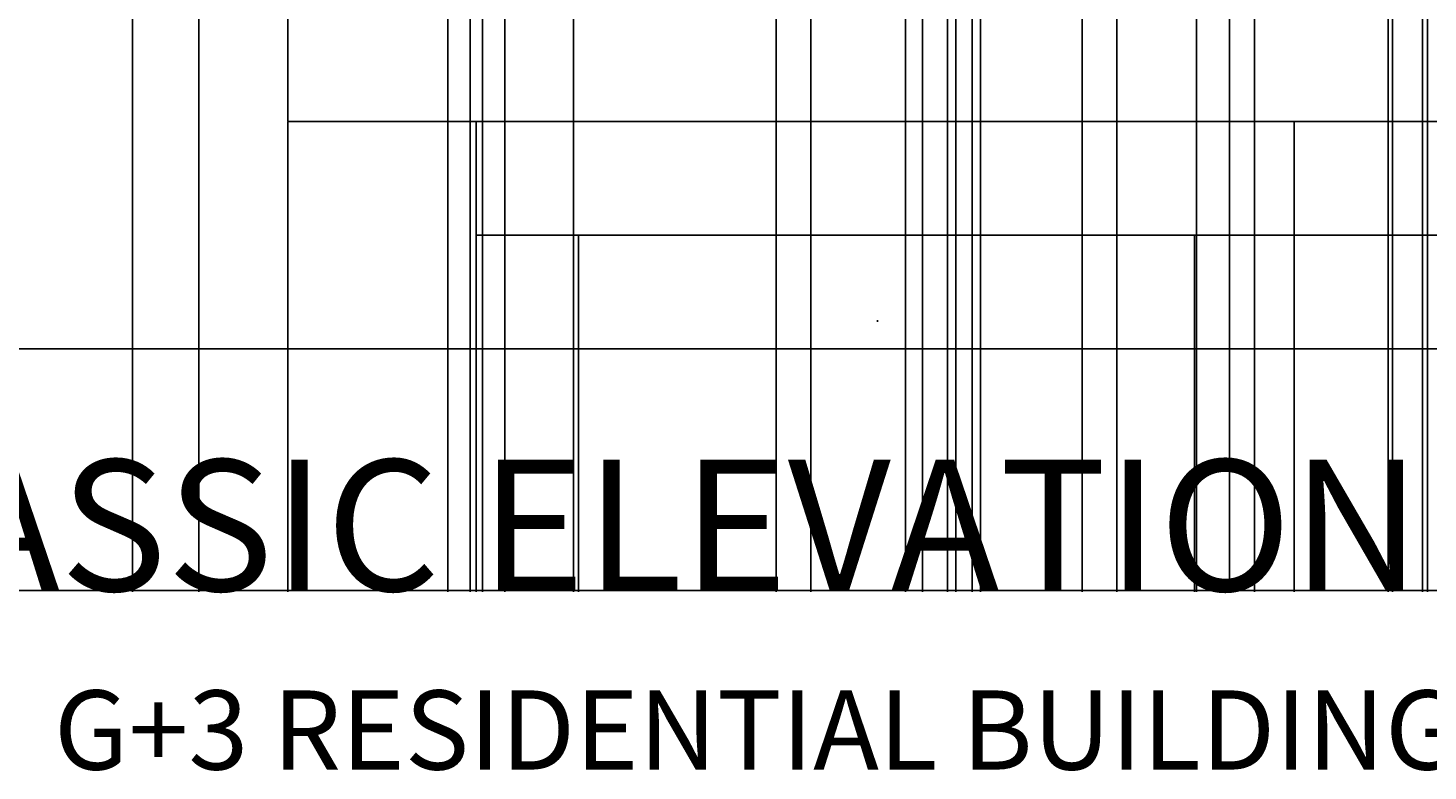
# Model space of a CAD drawing. Units: inches. Extents: x -14 to 375, y -86 to 549.
# Tile 2 of 12: x 122 to 290, y -86 to 4. Entities that reach past the tile are written whole.
import ezdxf

# ---------------------------------------------------------------- set-up
doc = ezdxf.new("R2010")
doc.units = ezdxf.units.IN
doc.header["$MEASUREMENT"] = 0
for name, color, linetype, lineweight in [('A-ANNO-DIMS', 2, 'Continuous', 18), ('A-ANNO-TEXT', 7, 'Continuous', 25), ('A-ELEV', 7, 'Continuous', 25)]:
    doc.layers.add(name, color=color, linetype=linetype, lineweight=lineweight)
doc.styles.get("Standard").update_dxf_attribs({"font": 'arial.ttf'})
doc.dimstyles.get("Standard").update_dxf_attribs({"dimtxt": 0.18, "dimasz": 0.18, "dimexe": 0.18, "dimexo": 0.0625, "dimgap": 0.09, "dimtad": 0, "dimtih": 1, "dimtoh": 1, "dimdec": 4, "dimzin": 0, "dimdsep": 46, "dimtxsty": 'Standard', "dimcen": 0.09, "dimadec": 0, "dimazin": 0, "dimtfac": 1, "dimtdec": 4, "dimtofl": 0, "dimtmove": 0, "dimatfit": 3, "dimfxl": 1, "dimtolj": 1, "dimtzin": 0, "dimarcsym": 0})

# ---------------------------------------------------------------- blocks, each defined once
blk = doc.blocks.new('*D4')
at = {"layer": 'A-ANNO-DIMS', "color": 0, "lineweight": -2, "transparency": 16777216}
for p, q in [((15.4, -35.17), (15.4, -64.39)), ((345.26, -35.17), (345.26, -64.39)), ((15.58, -64.21), (179.87, -64.21)), ((345.08, -64.21), (180.8, -64.21))]:
    blk.add_line(p, q, dxfattribs=at)
at = {"layer": 'A-ANNO-DIMS', "color": 0, "transparency": 16777216}
for points in [[(15.58, -64.18), (15.58, -64.24), (15.4, -64.21)], [(345.08, -64.18), (345.08, -64.24), (345.26, -64.21)]]:
    blk.add_solid(points, dxfattribs=at)
at = {"layer": 'Defpoints', "color": 0, "transparency": 16777216}
for p in [(15.4, -35.11), (345.26, -35.11), (345.26, -64.21)]:
    blk.add_point(p, dxfattribs=at)
at = {"layer": 'A-ANNO-DIMS', "color": 0, "transparency": 16777216, "insert": (180.33, -64.21), "char_height": 0.18, "attachment_point": 5}
blk.add_mtext('\\A1;329.86', dxfattribs=at)
blk = doc.blocks.new('*D42')
at = {"layer": 'A-ANNO-DIMS', "color": 0, "lineweight": -2, "transparency": 16777216}
for p, q in [((142.23, 270.64), (142.23, -64.39)), ((134.23, 262.64), (134.23, -64.39)), ((134.41, -64.21), (138.08, -64.21)), ((142.05, -64.21), (138.38, -64.21))]:
    blk.add_line(p, q, dxfattribs=at)
at = {"layer": 'A-ANNO-DIMS', "color": 0, "transparency": 16777216}
for points in [[(134.41, -64.18), (134.41, -64.24), (134.23, -64.21)], [(142.05, -64.18), (142.05, -64.24), (142.23, -64.21)]]:
    blk.add_solid(points, dxfattribs=at)
at = {"layer": 'Defpoints', "color": 0, "transparency": 16777216}
for p in [(142.23, 270.71), (134.23, 262.71), (142.23, -64.21)]:
    blk.add_point(p, dxfattribs=at)
at = {"layer": 'A-ANNO-DIMS', "color": 0, "transparency": 16777216, "insert": (138.23, -64.21), "char_height": 0.18, "attachment_point": 5}
blk.add_mtext('\\A1;8', dxfattribs=at)
blk = doc.blocks.new('*D43')
at = {"layer": 'A-ANNO-DIMS', "color": 0, "lineweight": -2, "transparency": 16777216}
for p, q in [((142.23, 270.64), (142.23, -64.39)), ((305.63, 270.64), (305.63, -64.39)), ((142.41, -64.21), (223.55, -64.21)), ((305.45, -64.21), (224.32, -64.21))]:
    blk.add_line(p, q, dxfattribs=at)
at = {"layer": 'A-ANNO-DIMS', "color": 0, "transparency": 16777216}
for points in [[(142.41, -64.18), (142.41, -64.24), (142.23, -64.21)], [(305.45, -64.18), (305.45, -64.24), (305.63, -64.21)]]:
    blk.add_solid(points, dxfattribs=at)
at = {"layer": 'Defpoints', "color": 0, "transparency": 16777216}
for p in [(142.23, 270.71), (305.63, 270.71), (305.63, -64.21)]:
    blk.add_point(p, dxfattribs=at)
at = {"layer": 'A-ANNO-DIMS', "color": 0, "transparency": 16777216, "insert": (223.93, -64.21), "char_height": 0.18, "attachment_point": 5}
blk.add_mtext('\\A1;163.4', dxfattribs=at)
blk = doc.blocks.new('*D45')
at = {"layer": 'A-ANNO-DIMS', "color": 0, "lineweight": -2, "transparency": 16777216}
for p, q in [((142.23, 306.64), (142.23, -64.39)), ((174.92, 306.64), (174.92, -64.39)), ((142.41, -64.21), (158.19, -64.21)), ((174.74, -64.21), (158.97, -64.21))]:
    blk.add_line(p, q, dxfattribs=at)
at = {"layer": 'A-ANNO-DIMS', "color": 0, "transparency": 16777216}
for points in [[(142.41, -64.18), (142.41, -64.24), (142.23, -64.21)], [(174.74, -64.18), (174.74, -64.24), (174.92, -64.21)]]:
    blk.add_solid(points, dxfattribs=at)
at = {"layer": 'Defpoints', "color": 0, "transparency": 16777216}
for p in [(142.23, 306.71), (174.92, 306.71), (174.92, -64.21)]:
    blk.add_point(p, dxfattribs=at)
at = {"layer": 'A-ANNO-DIMS', "color": 0, "transparency": 16777216, "insert": (158.58, -64.21), "char_height": 0.18, "attachment_point": 5}
blk.add_mtext('\\A1;32.69', dxfattribs=at)
blk = doc.blocks.new('*D46')
at = {"layer": 'A-ANNO-DIMS', "color": 0, "lineweight": -2, "transparency": 16777216}
for p, q in [((174.92, 306.64), (174.92, -64.39)), ((179.09, 306.64), (179.09, -64.39)), ((175.1, -64.21), (176.68, -64.21)), ((178.91, -64.21), (177.33, -64.21))]:
    blk.add_line(p, q, dxfattribs=at)
at = {"layer": 'A-ANNO-DIMS', "color": 0, "transparency": 16777216}
for points in [[(175.1, -64.18), (175.1, -64.24), (174.92, -64.21)], [(178.91, -64.18), (178.91, -64.24), (179.09, -64.21)]]:
    blk.add_solid(points, dxfattribs=at)
at = {"layer": 'Defpoints', "color": 0, "transparency": 16777216}
for p in [(174.92, 306.71), (179.09, 306.71), (179.09, -64.21)]:
    blk.add_point(p, dxfattribs=at)
at = {"layer": 'A-ANNO-DIMS', "color": 0, "transparency": 16777216, "insert": (177.01, -64.21), "char_height": 0.18, "attachment_point": 5}
blk.add_mtext('\\A1;4.17', dxfattribs=at)
blk = doc.blocks.new('*D47')
at = {"layer": 'A-ANNO-DIMS', "color": 0, "lineweight": -2, "transparency": 16777216}
for p, q in [((179.09, 306.64), (179.09, -64.39)), ((211.78, 306.64), (211.78, -64.39)), ((179.27, -64.21), (195.04, -64.21)), ((211.6, -64.21), (195.83, -64.21))]:
    blk.add_line(p, q, dxfattribs=at)
at = {"layer": 'A-ANNO-DIMS', "color": 0, "transparency": 16777216}
for points in [[(179.27, -64.18), (179.27, -64.24), (179.09, -64.21)], [(211.6, -64.18), (211.6, -64.24), (211.78, -64.21)]]:
    blk.add_solid(points, dxfattribs=at)
at = {"layer": 'Defpoints', "color": 0, "transparency": 16777216}
for p in [(179.09, 306.71), (211.78, 306.71), (211.78, -64.21)]:
    blk.add_point(p, dxfattribs=at)
at = {"layer": 'A-ANNO-DIMS', "color": 0, "transparency": 16777216, "insert": (195.44, -64.21), "char_height": 0.18, "attachment_point": 5}
blk.add_mtext('\\A1;32.69', dxfattribs=at)
blk = doc.blocks.new('*D48')
at = {"layer": 'A-ANNO-DIMS', "color": 0, "lineweight": -2, "transparency": 16777216}
for p, q in [((211.78, 306.64), (211.78, -64.39)), ((215.95, 306.64), (215.95, -64.39)), ((211.96, -64.21), (213.54, -64.21)), ((215.77, -64.21), (214.19, -64.21))]:
    blk.add_line(p, q, dxfattribs=at)
at = {"layer": 'A-ANNO-DIMS', "color": 0, "transparency": 16777216}
for points in [[(211.96, -64.18), (211.96, -64.24), (211.78, -64.21)], [(215.77, -64.18), (215.77, -64.24), (215.95, -64.21)]]:
    blk.add_solid(points, dxfattribs=at)
at = {"layer": 'Defpoints', "color": 0, "transparency": 16777216}
for p in [(211.78, 306.71), (215.95, 306.71), (215.95, -64.21)]:
    blk.add_point(p, dxfattribs=at)
at = {"layer": 'A-ANNO-DIMS', "color": 0, "transparency": 16777216, "insert": (213.86, -64.21), "char_height": 0.18, "attachment_point": 5}
blk.add_mtext('\\A1;4.17', dxfattribs=at)
blk = doc.blocks.new('*D49')
at = {"layer": 'A-ANNO-DIMS', "color": 0, "lineweight": -2, "transparency": 16777216}
for p, q in [((215.95, 306.64), (215.95, -64.39)), ((248.64, 306.64), (248.64, -64.39)), ((216.13, -64.21), (231.9, -64.21)), ((248.46, -64.21), (232.69, -64.21))]:
    blk.add_line(p, q, dxfattribs=at)
at = {"layer": 'A-ANNO-DIMS', "color": 0, "transparency": 16777216}
for points in [[(216.13, -64.18), (216.13, -64.24), (215.95, -64.21)], [(248.46, -64.18), (248.46, -64.24), (248.64, -64.21)]]:
    blk.add_solid(points, dxfattribs=at)
at = {"layer": 'Defpoints', "color": 0, "transparency": 16777216}
for p in [(215.95, 306.71), (248.64, 306.71), (248.64, -64.21)]:
    blk.add_point(p, dxfattribs=at)
at = {"layer": 'A-ANNO-DIMS', "color": 0, "transparency": 16777216, "insert": (232.29, -64.21), "char_height": 0.18, "attachment_point": 5}
blk.add_mtext('\\A1;32.69', dxfattribs=at)
blk = doc.blocks.new('*D50')
at = {"layer": 'A-ANNO-DIMS', "color": 0, "lineweight": -2, "transparency": 16777216}
for p, q in [((248.64, 306.64), (248.64, -64.39)), ((252.81, 306.64), (252.81, -64.39)), ((248.82, -64.21), (250.39, -64.21)), ((252.63, -64.21), (251.05, -64.21))]:
    blk.add_line(p, q, dxfattribs=at)
at = {"layer": 'A-ANNO-DIMS', "color": 0, "transparency": 16777216}
for points in [[(248.82, -64.18), (248.82, -64.24), (248.64, -64.21)], [(252.63, -64.18), (252.63, -64.24), (252.81, -64.21)]]:
    blk.add_solid(points, dxfattribs=at)
at = {"layer": 'Defpoints', "color": 0, "transparency": 16777216}
for p in [(248.64, 306.71), (252.81, 306.71), (252.81, -64.21)]:
    blk.add_point(p, dxfattribs=at)
at = {"layer": 'A-ANNO-DIMS', "color": 0, "transparency": 16777216, "insert": (250.72, -64.21), "char_height": 0.18, "attachment_point": 5}
blk.add_mtext('\\A1;4.17', dxfattribs=at)
blk = doc.blocks.new('*D51')
at = {"layer": 'A-ANNO-DIMS', "color": 0, "lineweight": -2, "transparency": 16777216}
for p, q in [((252.81, 306.64), (252.81, -64.39)), ((285.5, 306.64), (285.5, -64.39)), ((252.99, -64.21), (268.76, -64.21)), ((285.32, -64.21), (269.54, -64.21))]:
    blk.add_line(p, q, dxfattribs=at)
at = {"layer": 'A-ANNO-DIMS', "color": 0, "transparency": 16777216}
for points in [[(252.99, -64.18), (252.99, -64.24), (252.81, -64.21)], [(285.32, -64.18), (285.32, -64.24), (285.5, -64.21)]]:
    blk.add_solid(points, dxfattribs=at)
at = {"layer": 'Defpoints', "color": 0, "transparency": 16777216}
for p in [(252.81, 306.71), (285.5, 306.71), (285.5, -64.21)]:
    blk.add_point(p, dxfattribs=at)
at = {"layer": 'A-ANNO-DIMS', "color": 0, "transparency": 16777216, "insert": (269.15, -64.21), "char_height": 0.18, "attachment_point": 5}
blk.add_mtext('\\A1;32.69', dxfattribs=at)
blk = doc.blocks.new('*D52')
at = {"layer": 'A-ANNO-DIMS', "color": 0, "lineweight": -2, "transparency": 16777216}
for p, q in [((285.5, 306.64), (285.5, -64.39)), ((289.66, 306.64), (289.66, -64.39)), ((285.68, -64.21), (287.25, -64.21)), ((289.48, -64.21), (287.91, -64.21))]:
    blk.add_line(p, q, dxfattribs=at)
at = {"layer": 'A-ANNO-DIMS', "color": 0, "transparency": 16777216}
for points in [[(285.68, -64.18), (285.68, -64.24), (285.5, -64.21)], [(289.48, -64.18), (289.48, -64.24), (289.66, -64.21)]]:
    blk.add_solid(points, dxfattribs=at)
at = {"layer": 'Defpoints', "color": 0, "transparency": 16777216}
for p in [(285.5, 306.71), (289.66, 306.71), (289.66, -64.21)]:
    blk.add_point(p, dxfattribs=at)
at = {"layer": 'A-ANNO-DIMS', "color": 0, "transparency": 16777216, "insert": (287.58, -64.21), "char_height": 0.18, "attachment_point": 5}
blk.add_mtext('\\A1;4.17', dxfattribs=at)
blk = doc.blocks.new('*D57')
at = {"layer": 'A-ANNO-DIMS', "color": 0, "lineweight": -2, "transparency": 16777216}
for p, q in [((229.41, 340.38), (229.41, -64.39)), ((232.41, 340.38), (232.41, -64.39)), ((229.59, -64.21), (230.76, -64.21)), ((232.23, -64.21), (231.06, -64.21))]:
    blk.add_line(p, q, dxfattribs=at)
at = {"layer": 'A-ANNO-DIMS', "color": 0, "transparency": 16777216}
for points in [[(229.59, -64.18), (229.59, -64.24), (229.41, -64.21)], [(232.23, -64.18), (232.23, -64.24), (232.41, -64.21)]]:
    blk.add_solid(points, dxfattribs=at)
at = {"layer": 'Defpoints', "color": 0, "transparency": 16777216}
for p in [(229.41, 340.44), (232.41, 340.44), (232.41, -64.21)]:
    blk.add_point(p, dxfattribs=at)
at = {"layer": 'A-ANNO-DIMS', "color": 0, "transparency": 16777216, "insert": (230.91, -64.21), "char_height": 0.18, "attachment_point": 5}
blk.add_mtext('\\A1;3', dxfattribs=at)
blk = doc.blocks.new('*D58')
at = {"layer": 'A-ANNO-DIMS', "color": 0, "lineweight": -2, "transparency": 16777216}
for p, q in [((232.41, 340.38), (232.41, -64.39)), ((236.41, 340.38), (236.41, -64.39)), ((232.59, -64.21), (234.26, -64.21)), ((236.23, -64.21), (234.56, -64.21))]:
    blk.add_line(p, q, dxfattribs=at)
at = {"layer": 'A-ANNO-DIMS', "color": 0, "transparency": 16777216}
for points in [[(232.59, -64.18), (232.59, -64.24), (232.41, -64.21)], [(236.23, -64.18), (236.23, -64.24), (236.41, -64.21)]]:
    blk.add_solid(points, dxfattribs=at)
at = {"layer": 'Defpoints', "color": 0, "transparency": 16777216}
for p in [(232.41, 340.44), (236.41, 340.44), (236.41, -64.21)]:
    blk.add_point(p, dxfattribs=at)
at = {"layer": 'A-ANNO-DIMS', "color": 0, "transparency": 16777216, "insert": (234.41, -64.21), "char_height": 0.18, "attachment_point": 5}
blk.add_mtext('\\A1;4', dxfattribs=at)
blk = doc.blocks.new('*D59')
at = {"layer": 'A-ANNO-DIMS', "color": 0, "lineweight": -2, "transparency": 16777216}
for p, q in [((236.41, 340.38), (236.41, -64.39)), ((262.41, 340.38), (262.41, -64.39)), ((236.59, -64.21), (249.19, -64.21)), ((262.23, -64.21), (249.63, -64.21))]:
    blk.add_line(p, q, dxfattribs=at)
at = {"layer": 'A-ANNO-DIMS', "color": 0, "transparency": 16777216}
for points in [[(236.59, -64.18), (236.59, -64.24), (236.41, -64.21)], [(262.23, -64.18), (262.23, -64.24), (262.41, -64.21)]]:
    blk.add_solid(points, dxfattribs=at)
at = {"layer": 'Defpoints', "color": 0, "transparency": 16777216}
for p in [(236.41, 340.44), (262.41, 340.44), (262.41, -64.21)]:
    blk.add_point(p, dxfattribs=at)
at = {"layer": 'A-ANNO-DIMS', "color": 0, "transparency": 16777216, "insert": (249.41, -64.21), "char_height": 0.18, "attachment_point": 5}
blk.add_mtext('\\A1;26', dxfattribs=at)
blk = doc.blocks.new('*D60')
at = {"layer": 'A-ANNO-DIMS', "color": 0, "lineweight": -2, "transparency": 16777216}
for p, q in [((262.41, 340.38), (262.41, -64.39)), ((266.41, 340.38), (266.41, -64.39)), ((262.59, -64.21), (264.26, -64.21)), ((266.23, -64.21), (264.56, -64.21))]:
    blk.add_line(p, q, dxfattribs=at)
at = {"layer": 'A-ANNO-DIMS', "color": 0, "transparency": 16777216}
for points in [[(262.59, -64.18), (262.59, -64.24), (262.41, -64.21)], [(266.23, -64.18), (266.23, -64.24), (266.41, -64.21)]]:
    blk.add_solid(points, dxfattribs=at)
at = {"layer": 'Defpoints', "color": 0, "transparency": 16777216}
for p in [(262.41, 340.44), (266.41, 340.44), (266.41, -64.21)]:
    blk.add_point(p, dxfattribs=at)
at = {"layer": 'A-ANNO-DIMS', "color": 0, "transparency": 16777216, "insert": (264.41, -64.21), "char_height": 0.18, "attachment_point": 5}
blk.add_mtext('\\A1;4', dxfattribs=at)
blk = doc.blocks.new('*D61')
at = {"layer": 'A-ANNO-DIMS', "color": 0, "lineweight": -2, "transparency": 16777216}
for p, q in [((266.41, 340.38), (266.41, -64.39)), ((269.41, 340.38), (269.41, -64.39)), ((266.59, -64.21), (267.76, -64.21)), ((269.23, -64.21), (268.06, -64.21))]:
    blk.add_line(p, q, dxfattribs=at)
at = {"layer": 'A-ANNO-DIMS', "color": 0, "transparency": 16777216}
for points in [[(266.59, -64.18), (266.59, -64.24), (266.41, -64.21)], [(269.23, -64.18), (269.23, -64.24), (269.41, -64.21)]]:
    blk.add_solid(points, dxfattribs=at)
at = {"layer": 'Defpoints', "color": 0, "transparency": 16777216}
for p in [(266.41, 340.44), (269.41, 340.44), (269.41, -64.21)]:
    blk.add_point(p, dxfattribs=at)
at = {"layer": 'A-ANNO-DIMS', "color": 0, "transparency": 16777216, "insert": (267.91, -64.21), "char_height": 0.18, "attachment_point": 5}
blk.add_mtext('\\A1;3', dxfattribs=at)
blk = doc.blocks.new('*D71')
at = {"layer": 'A-ANNO-DIMS', "color": 0, "lineweight": -2, "transparency": 16777216}
for p, q in [((233.41, 167.91), (233.41, -64.39)), ((235.41, 167.91), (235.41, -64.39)), ((233.59, -64.21), (234.26, -64.21)), ((235.23, -64.21), (234.56, -64.21))]:
    blk.add_line(p, q, dxfattribs=at)
at = {"layer": 'A-ANNO-DIMS', "color": 0, "transparency": 16777216}
for points in [[(233.59, -64.18), (233.59, -64.24), (233.41, -64.21)], [(235.23, -64.18), (235.23, -64.24), (235.41, -64.21)]]:
    blk.add_solid(points, dxfattribs=at)
at = {"layer": 'Defpoints', "color": 0, "transparency": 16777216}
for p in [(233.41, 167.97), (235.41, 167.97), (235.41, -64.21)]:
    blk.add_point(p, dxfattribs=at)
at = {"layer": 'A-ANNO-DIMS', "color": 0, "transparency": 16777216, "insert": (234.41, -64.21), "char_height": 0.18, "attachment_point": 5}
blk.add_mtext('\\A1;2', dxfattribs=at)
blk = doc.blocks.new('*D74')
at = {"layer": 'A-ANNO-DIMS', "color": 0, "lineweight": -2, "transparency": 16777216}
for p, q in [((142.23, 125.9), (142.23, -64.39)), ((134.23, 117.9), (134.23, -64.39)), ((134.41, -64.21), (138.08, -64.21)), ((142.05, -64.21), (138.38, -64.21))]:
    blk.add_line(p, q, dxfattribs=at)
at = {"layer": 'A-ANNO-DIMS', "color": 0, "transparency": 16777216}
for points in [[(134.41, -64.18), (134.41, -64.24), (134.23, -64.21)], [(142.05, -64.18), (142.05, -64.24), (142.23, -64.21)]]:
    blk.add_solid(points, dxfattribs=at)
at = {"layer": 'Defpoints', "color": 0, "transparency": 16777216}
for p in [(142.23, 125.96), (134.23, 117.96), (142.23, -64.21)]:
    blk.add_point(p, dxfattribs=at)
at = {"layer": 'A-ANNO-DIMS', "color": 0, "transparency": 16777216, "insert": (138.23, -64.21), "char_height": 0.18, "attachment_point": 5}
blk.add_mtext('\\A1;8', dxfattribs=at)
blk = doc.blocks.new('*D75')
at = {"layer": 'A-ANNO-DIMS', "color": 0, "lineweight": -2, "transparency": 16777216}
for p, q in [((142.23, 125.9), (142.23, -64.39)), ((172.23, 125.9), (172.23, -64.39)), ((142.41, -64.21), (157.01, -64.21)), ((172.05, -64.21), (157.45, -64.21))]:
    blk.add_line(p, q, dxfattribs=at)
at = {"layer": 'A-ANNO-DIMS', "color": 0, "transparency": 16777216}
for points in [[(142.41, -64.18), (142.41, -64.24), (142.23, -64.21)], [(172.05, -64.18), (172.05, -64.24), (172.23, -64.21)]]:
    blk.add_solid(points, dxfattribs=at)
at = {"layer": 'Defpoints', "color": 0, "transparency": 16777216}
for p in [(142.23, 125.96), (172.23, 125.96), (172.23, -64.21)]:
    blk.add_point(p, dxfattribs=at)
at = {"layer": 'A-ANNO-DIMS', "color": 0, "transparency": 16777216, "insert": (157.23, -64.21), "char_height": 0.18, "attachment_point": 5}
blk.add_mtext('\\A1;30', dxfattribs=at)
blk = doc.blocks.new('*D76')
at = {"layer": 'A-ANNO-DIMS', "color": 0, "lineweight": -2, "transparency": 16777216}
for p, q in [((172.23, 125.9), (172.23, -64.39)), ((176.42, 125.9), (176.42, -64.39)), ((172.41, -64.21), (173.93, -64.21)), ((176.24, -64.21), (174.72, -64.21))]:
    blk.add_line(p, q, dxfattribs=at)
at = {"layer": 'A-ANNO-DIMS', "color": 0, "transparency": 16777216}
for points in [[(172.41, -64.18), (172.41, -64.24), (172.23, -64.21)], [(176.24, -64.18), (176.24, -64.24), (176.42, -64.21)]]:
    blk.add_solid(points, dxfattribs=at)
at = {"layer": 'Defpoints', "color": 0, "transparency": 16777216}
for p in [(172.23, 125.96), (176.42, 125.96), (176.42, -64.21)]:
    blk.add_point(p, dxfattribs=at)
at = {"layer": 'A-ANNO-DIMS', "color": 0, "transparency": 16777216, "insert": (174.32, -64.21), "char_height": 0.18, "attachment_point": 5}
blk.add_mtext('\\A1;4.186', dxfattribs=at)
blk = doc.blocks.new('*D77')
at = {"layer": 'A-ANNO-DIMS', "color": 0, "lineweight": -2, "transparency": 16777216}
for p, q in [((176.42, 125.9), (176.42, -64.39)), ((187.37, 125.91), (187.37, -64.39)), ((176.6, -64.21), (181.44, -64.21)), ((187.19, -64.21), (182.35, -64.21))]:
    blk.add_line(p, q, dxfattribs=at)
at = {"layer": 'A-ANNO-DIMS', "color": 0, "transparency": 16777216}
for points in [[(176.6, -64.18), (176.6, -64.24), (176.42, -64.21)], [(187.19, -64.18), (187.19, -64.24), (187.37, -64.21)]]:
    blk.add_solid(points, dxfattribs=at)
at = {"layer": 'Defpoints', "color": 0, "transparency": 16777216}
for p in [(176.42, 125.96), (187.37, 125.97), (187.37, -64.21)]:
    blk.add_point(p, dxfattribs=at)
at = {"layer": 'A-ANNO-DIMS', "color": 0, "transparency": 16777216, "insert": (181.89, -64.21), "char_height": 0.18, "attachment_point": 5}
blk.add_mtext('\\A1;10.949', dxfattribs=at)
blk = doc.blocks.new('*D78')
at = {"layer": 'A-ANNO-DIMS', "color": 0, "lineweight": -2, "transparency": 16777216}
for p, q in [((187.37, 125.91), (187.37, -64.39)), ((227.37, 125.91), (227.37, -64.39)), ((187.55, -64.21), (207.14, -64.21)), ((227.19, -64.21), (207.59, -64.21))]:
    blk.add_line(p, q, dxfattribs=at)
at = {"layer": 'A-ANNO-DIMS', "color": 0, "transparency": 16777216}
for points in [[(187.55, -64.18), (187.55, -64.24), (187.37, -64.21)], [(227.19, -64.18), (227.19, -64.24), (227.37, -64.21)]]:
    blk.add_solid(points, dxfattribs=at)
at = {"layer": 'Defpoints', "color": 0, "transparency": 16777216}
for p in [(187.37, 125.97), (227.37, 125.97), (227.37, -64.21)]:
    blk.add_point(p, dxfattribs=at)
at = {"layer": 'A-ANNO-DIMS', "color": 0, "transparency": 16777216, "insert": (207.37, -64.21), "char_height": 0.18, "attachment_point": 5}
blk.add_mtext('\\A1;40', dxfattribs=at)
blk = doc.blocks.new('*D79')
at = {"layer": 'A-ANNO-DIMS', "color": 0, "lineweight": -2, "transparency": 16777216}
for p, q in [((227.37, 125.91), (227.37, -64.39)), ((229.41, 125.91), (229.41, -64.39)), ((227.55, -64.21), (228.06, -64.21)), ((229.23, -64.21), (228.71, -64.21))]:
    blk.add_line(p, q, dxfattribs=at)
at = {"layer": 'A-ANNO-DIMS', "color": 0, "transparency": 16777216}
for points in [[(227.55, -64.18), (227.55, -64.24), (227.37, -64.21)], [(229.23, -64.18), (229.23, -64.24), (229.41, -64.21)]]:
    blk.add_solid(points, dxfattribs=at)
at = {"layer": 'Defpoints', "color": 0, "transparency": 16777216}
for p in [(227.37, 125.97), (229.41, 125.97), (229.41, -64.21)]:
    blk.add_point(p, dxfattribs=at)
at = {"layer": 'A-ANNO-DIMS', "color": 0, "transparency": 16777216, "insert": (228.39, -64.21), "char_height": 0.18, "attachment_point": 5}
blk.add_mtext('\\A1;2.04', dxfattribs=at)
blk = doc.blocks.new('*D80')
at = {"layer": 'A-ANNO-DIMS', "color": 0, "lineweight": -2, "transparency": 16777216}
for p, q in [((229.41, 125.91), (229.41, -64.39)), ((269.41, 125.91), (269.41, -64.39)), ((229.59, -64.21), (249.19, -64.21)), ((269.23, -64.21), (249.63, -64.21))]:
    blk.add_line(p, q, dxfattribs=at)
at = {"layer": 'A-ANNO-DIMS', "color": 0, "transparency": 16777216}
for points in [[(229.59, -64.18), (229.59, -64.24), (229.41, -64.21)], [(269.23, -64.18), (269.23, -64.24), (269.41, -64.21)]]:
    blk.add_solid(points, dxfattribs=at)
at = {"layer": 'Defpoints', "color": 0, "transparency": 16777216}
for p in [(229.41, 125.97), (269.41, 125.97), (269.41, -64.21)]:
    blk.add_point(p, dxfattribs=at)
at = {"layer": 'A-ANNO-DIMS', "color": 0, "transparency": 16777216, "insert": (249.41, -64.21), "char_height": 0.18, "attachment_point": 5}
blk.add_mtext('\\A1;40', dxfattribs=at)
blk = doc.blocks.new('*D81')
at = {"layer": 'A-ANNO-DIMS', "color": 0, "lineweight": -2, "transparency": 16777216}
for p, q in [((269.41, 125.91), (269.41, -64.39)), ((286.05, 125.9), (286.05, -64.39)), ((269.59, -64.21), (277.34, -64.21)), ((285.87, -64.21), (278.11, -64.21))]:
    blk.add_line(p, q, dxfattribs=at)
at = {"layer": 'A-ANNO-DIMS', "color": 0, "transparency": 16777216}
for points in [[(269.59, -64.18), (269.59, -64.24), (269.41, -64.21)], [(285.87, -64.18), (285.87, -64.24), (286.05, -64.21)]]:
    blk.add_solid(points, dxfattribs=at)
at = {"layer": 'Defpoints', "color": 0, "transparency": 16777216}
for p in [(269.41, 125.97), (286.05, 125.96), (286.05, -64.21)]:
    blk.add_point(p, dxfattribs=at)
at = {"layer": 'A-ANNO-DIMS', "color": 0, "transparency": 16777216, "insert": (277.73, -64.21), "char_height": 0.18, "attachment_point": 5}
blk.add_mtext('\\A1;16.64', dxfattribs=at)
blk = doc.blocks.new('*D82')
at = {"layer": 'A-ANNO-DIMS', "color": 0, "lineweight": -2, "transparency": 16777216}
for p, q in [((286.05, 125.9), (286.05, -64.39)), ((290.24, 125.9), (290.24, -64.39)), ((286.23, -64.21), (287.75, -64.21)), ((290.06, -64.21), (288.54, -64.21))]:
    blk.add_line(p, q, dxfattribs=at)
at = {"layer": 'A-ANNO-DIMS', "color": 0, "transparency": 16777216}
for points in [[(286.23, -64.18), (286.23, -64.24), (286.05, -64.21)], [(290.06, -64.18), (290.06, -64.24), (290.24, -64.21)]]:
    blk.add_solid(points, dxfattribs=at)
at = {"layer": 'Defpoints', "color": 0, "transparency": 16777216}
for p in [(286.05, 125.96), (290.24, 125.96), (290.24, -64.21)]:
    blk.add_point(p, dxfattribs=at)
at = {"layer": 'A-ANNO-DIMS', "color": 0, "transparency": 16777216, "insert": (288.14, -64.21), "char_height": 0.18, "attachment_point": 5}
blk.add_mtext('\\A1;4.186', dxfattribs=at)
blk = doc.blocks.new('*D83')
at = {"layer": 'A-ANNO-DIMS', "color": 0, "lineweight": -2, "transparency": 16777216}
for p, q in [((290.24, 125.9), (290.24, -64.39)), ((305.77, 125.9), (305.77, -64.39)), ((290.42, -64.21), (297.55, -64.21)), ((305.59, -64.21), (298.46, -64.21))]:
    blk.add_line(p, q, dxfattribs=at)
at = {"layer": 'A-ANNO-DIMS', "color": 0, "transparency": 16777216}
for points in [[(290.42, -64.18), (290.42, -64.24), (290.24, -64.21)], [(305.59, -64.18), (305.59, -64.24), (305.77, -64.21)]]:
    blk.add_solid(points, dxfattribs=at)
at = {"layer": 'Defpoints', "color": 0, "transparency": 16777216}
for p in [(290.24, 125.96), (305.77, 125.96), (305.77, -64.21)]:
    blk.add_point(p, dxfattribs=at)
at = {"layer": 'A-ANNO-DIMS', "color": 0, "transparency": 16777216, "insert": (298, -64.21), "char_height": 0.18, "attachment_point": 5}
blk.add_mtext('\\A1;15.534', dxfattribs=at)
blk = doc.blocks.new('*D108')
at = {"layer": 'A-ANNO-DIMS', "color": 0, "lineweight": -2, "transparency": 16777216}
for p, q in [((134.23, 5.9), (134.23, -64.39)), ((152.96, -7.79), (152.96, -64.39)), ((134.41, -64.21), (143.21, -64.21)), ((152.78, -64.21), (143.98, -64.21))]:
    blk.add_line(p, q, dxfattribs=at)
at = {"layer": 'A-ANNO-DIMS', "color": 0, "transparency": 16777216}
for points in [[(134.41, -64.18), (134.41, -64.24), (134.23, -64.21)], [(152.78, -64.18), (152.78, -64.24), (152.96, -64.21)]]:
    blk.add_solid(points, dxfattribs=at)
at = {"layer": 'Defpoints', "color": 0, "transparency": 16777216}
for p in [(134.23, 5.96), (152.96, -7.73), (152.96, -64.21)]:
    blk.add_point(p, dxfattribs=at)
at = {"layer": 'A-ANNO-DIMS', "color": 0, "transparency": 16777216, "insert": (143.6, -64.21), "char_height": 0.18, "attachment_point": 5}
blk.add_mtext('\\A1;18.73', dxfattribs=at)
blk = doc.blocks.new('*D109')
at = {"layer": 'A-ANNO-DIMS', "color": 0, "lineweight": -2, "transparency": 16777216}
for p, q in [((152.96, -7.79), (152.96, -64.39)), ((297.19, -7.79), (297.19, -64.39)), ((153.14, -64.21), (224.62, -64.21)), ((297.01, -64.21), (225.53, -64.21))]:
    blk.add_line(p, q, dxfattribs=at)
at = {"layer": 'A-ANNO-DIMS', "color": 0, "transparency": 16777216}
for points in [[(153.14, -64.18), (153.14, -64.24), (152.96, -64.21)], [(297.01, -64.18), (297.01, -64.24), (297.19, -64.21)]]:
    blk.add_solid(points, dxfattribs=at)
at = {"layer": 'Defpoints', "color": 0, "transparency": 16777216}
for p in [(152.96, -7.73), (297.19, -7.73), (297.19, -64.21)]:
    blk.add_point(p, dxfattribs=at)
at = {"layer": 'A-ANNO-DIMS', "color": 0, "transparency": 16777216, "insert": (225.08, -64.21), "char_height": 0.18, "attachment_point": 5}
blk.add_mtext('\\A1;144.23', dxfattribs=at)
blk = doc.blocks.new('*D110')
at = {"layer": 'A-ANNO-DIMS', "color": 0, "lineweight": -2, "transparency": 16777216}
for p, q in [((175.63, -21.48), (175.63, -64.39)), ((274.19, -21.48), (274.19, -64.39)), ((175.81, -64.21), (224.52, -64.21)), ((274.01, -64.21), (225.3, -64.21))]:
    blk.add_line(p, q, dxfattribs=at)
at = {"layer": 'A-ANNO-DIMS', "color": 0, "transparency": 16777216}
for points in [[(175.81, -64.18), (175.81, -64.24), (175.63, -64.21)], [(274.01, -64.18), (274.01, -64.24), (274.19, -64.21)]]:
    blk.add_solid(points, dxfattribs=at)
at = {"layer": 'Defpoints', "color": 0, "transparency": 16777216}
for p in [(175.63, -21.42), (274.19, -21.42), (274.19, -64.21)]:
    blk.add_point(p, dxfattribs=at)
at = {"layer": 'A-ANNO-DIMS', "color": 0, "transparency": 16777216, "insert": (224.91, -64.21), "char_height": 0.18, "attachment_point": 5}
blk.add_mtext('\\A1;98.57', dxfattribs=at)
blk = doc.blocks.new('*D111')
at = {"layer": 'A-ANNO-DIMS', "color": 0, "lineweight": -2, "transparency": 16777216}
for p, q in [((187.96, -35.17), (187.96, -64.39)), ((262.19, -35.17), (262.19, -64.39)), ((188.14, -64.21), (224.69, -64.21)), ((262.01, -64.21), (225.47, -64.21))]:
    blk.add_line(p, q, dxfattribs=at)
at = {"layer": 'A-ANNO-DIMS', "color": 0, "transparency": 16777216}
for points in [[(188.14, -64.18), (188.14, -64.24), (187.96, -64.21)], [(262.01, -64.18), (262.01, -64.24), (262.19, -64.21)]]:
    blk.add_solid(points, dxfattribs=at)
at = {"layer": 'Defpoints', "color": 0, "transparency": 16777216}
for p in [(187.96, -35.11), (262.19, -35.11), (262.19, -64.21)]:
    blk.add_point(p, dxfattribs=at)
at = {"layer": 'A-ANNO-DIMS', "color": 0, "transparency": 16777216, "insert": (225.08, -64.21), "char_height": 0.18, "attachment_point": 5}
blk.add_mtext('\\A1;74.23', dxfattribs=at)
blk = doc.blocks.new('*D113')
at = {"layer": 'A-ANNO-DIMS', "color": 0, "lineweight": -2, "transparency": 16777216}
for p, q in [((297.26, -7.73), (374.54, -7.73)), ((374.36, -7.91), (374.36, -14.39)), ((374.36, -21.24), (374.36, -14.76)), ((274.26, -21.42), (374.54, -21.42))]:
    blk.add_line(p, q, dxfattribs=at)
at = {"layer": 'A-ANNO-DIMS', "color": 0, "transparency": 16777216}
for points in [[(374.33, -7.91), (374.39, -7.91), (374.36, -7.73)], [(374.33, -21.24), (374.39, -21.24), (374.36, -21.42)]]:
    blk.add_solid(points, dxfattribs=at)
at = {"layer": 'Defpoints', "color": 0, "transparency": 16777216}
for p in [(297.19, -7.73), (274.19, -21.42), (374.36, -21.42)]:
    blk.add_point(p, dxfattribs=at)
at = {"layer": 'A-ANNO-DIMS', "color": 0, "transparency": 16777216, "insert": (374.36, -14.58), "char_height": 0.18, "attachment_point": 5}
blk.add_mtext('\\A1;13.69', dxfattribs=at)
blk = doc.blocks.new('*D114')
at = {"layer": 'A-ANNO-DIMS', "color": 0, "lineweight": -2, "transparency": 16777216}
for p, q in [((274.26, -21.42), (374.54, -21.42)), ((374.36, -21.6), (374.36, -28.08)), ((374.36, -34.93), (374.36, -28.45)), ((262.26, -35.11), (374.54, -35.11))]:
    blk.add_line(p, q, dxfattribs=at)
at = {"layer": 'A-ANNO-DIMS', "color": 0, "transparency": 16777216}
for points in [[(374.33, -21.6), (374.39, -21.6), (374.36, -21.42)], [(374.33, -34.93), (374.39, -34.93), (374.36, -35.11)]]:
    blk.add_solid(points, dxfattribs=at)
at = {"layer": 'Defpoints', "color": 0, "transparency": 16777216}
for p in [(274.19, -21.42), (262.19, -35.11), (374.36, -35.11)]:
    blk.add_point(p, dxfattribs=at)
at = {"layer": 'A-ANNO-DIMS', "color": 0, "transparency": 16777216, "insert": (374.36, -28.27), "char_height": 0.18, "attachment_point": 5}
blk.add_mtext('\\A1;13.69', dxfattribs=at)
blk = doc.blocks.new('*D137')
at = {"layer": 'A-ANNO-DIMS', "color": 0, "lineweight": -2, "transparency": 16777216}
for p, q in [((224.18, 189.18), (224, 189.18)), ((224, 189.18), (224, 106.51)), ((223.91, -31.75), (224.09, -31.75)), ((224, -31.84), (224, -31.66))]:
    blk.add_line(p, q, dxfattribs=at)
at = {"layer": 'A-ANNO-DIMS', "color": 0, "transparency": 16777216}
blk.add_solid([(223.97, 106.51), (224.03, 106.51), (224, 106.33)], dxfattribs=at)
at = {"layer": 'Defpoints', "color": 0, "transparency": 16777216}
for p in [(224, 106.33), (224, -31.75)]:
    blk.add_point(p, dxfattribs=at)
at = {"layer": 'A-ANNO-DIMS', "color": 0, "transparency": 16777216, "insert": (224.73, 189.18), "char_height": 0.18, "attachment_point": 5}
blk.add_mtext('\\A1;R138.08', dxfattribs=at)
blk = doc.blocks.new('*D138')
at = {"layer": 'A-ANNO-DIMS', "color": 0, "lineweight": -2, "transparency": 16777216}
for p, q in [((224.18, 176.38), (224, 176.38)), ((224, 176.38), (224, 98.51)), ((223.91, -31.75), (224.09, -31.75)), ((224, -31.84), (224, -31.66))]:
    blk.add_line(p, q, dxfattribs=at)
at = {"layer": 'A-ANNO-DIMS', "color": 0, "transparency": 16777216}
blk.add_solid([(223.97, 98.51), (224.03, 98.51), (224, 98.33)], dxfattribs=at)
at = {"layer": 'Defpoints', "color": 0, "transparency": 16777216}
for p in [(224, 98.33), (224, -31.75)]:
    blk.add_point(p, dxfattribs=at)
at = {"layer": 'A-ANNO-DIMS', "color": 0, "transparency": 16777216, "insert": (224.73, 176.38), "char_height": 0.18, "attachment_point": 5}
blk.add_mtext('\\A1;R130.08', dxfattribs=at)

msp = doc.modelspace()

# ---------------------------------------------------------------- linework, layer by layer
at = {"layer": 'A-ELEV'}
for points in [[(15.4018, 5.9589), (345.2647, 5.9589), (345.2647, -35.1115), (15.4018, -35.1115)], [(152.9633, 5.9589), (297.193, 5.9589), (297.193, -7.7312), (152.9633, -7.7312)], [(175.6275, -7.7312), (274.193, -7.7312), (274.193, -21.4214), (175.6275, -21.4214)], [(187.9633, -21.4214), (262.193, -21.4214), (262.193, -35.1115), (187.9633, -35.1115)]]:
    msp.add_lwpolyline(points, close=True, dxfattribs=at)

# ---------------------------------------------------------------- texts
at = {"layer": 'A-ANNO-TEXT'}
for s, height, p in [('CLASSIC ELEVATION', 15.79618, (86.9661, -64.2648)), ('G+3 RESIDENTIAL BUILDING', 9.539085, (124.7897, -85.7919))]:
    msp.add_text(s, height=height, dxfattribs=at).set_placement(p)

# ---------------------------------------------------------------- dimensions: what is measured, and where the dimension line sits
at = {"layer": 'A-ANNO-DIMS'}
for base, p1, p2, override, picture, middle in [((232.409, -64.2115), (229.409, 340.4421), (232.409, 340.4421), {"dimdec": 0, "dimlfac": 1, "dimrnd": 0, "dimzin": 0, "dimdsep": 46, "dimlunit": 2}, '*D57', (230.909, -64.2115)), ((236.409, -64.2115), (232.409, 340.4421), (236.409, 340.4421), {"dimdec": 0, "dimlfac": 1, "dimrnd": 0, "dimzin": 0, "dimdsep": 46, "dimlunit": 2}, '*D58', (234.409, -64.2115)), ((262.409, -64.2115), (236.409, 340.4421), (262.409, 340.4421), {"dimdec": 0, "dimlfac": 1, "dimrnd": 0, "dimzin": 0, "dimdsep": 46, "dimlunit": 2}, '*D59', (249.409, -64.2115)), ((266.409, -64.2115), (262.409, 340.4421), (266.409, 340.4421), {"dimdec": 0, "dimlfac": 1, "dimrnd": 0, "dimzin": 0, "dimdsep": 46, "dimlunit": 2}, '*D60', (264.409, -64.2115)), ((269.409, -64.2115), (266.409, 340.4421), (269.409, 340.4421), {"dimdec": 0, "dimlfac": 1, "dimrnd": 0, "dimzin": 0, "dimdsep": 46, "dimlunit": 2}, '*D61', (267.909, -64.2115)), ((174.9243, -64.2115), (142.2334, 306.7071), (174.9243, 306.7071), {"dimdec": 2, "dimlfac": 1, "dimrnd": 0, "dimzin": 0, "dimdsep": 46, "dimlunit": 2}, '*D45', (158.5788, -64.2115)), ((179.0907, -64.2115), (174.9243, 306.7071), (179.0907, 306.7071), {"dimdec": 2, "dimlfac": 1, "dimrnd": 0, "dimzin": 0, "dimdsep": 46, "dimlunit": 2}, '*D46', (177.0075, -64.2115)), ((211.7816, -64.2115), (179.0907, 306.7071), (211.7816, 306.7071), {"dimdec": 2, "dimlfac": 1, "dimrnd": 0, "dimzin": 0, "dimdsep": 46, "dimlunit": 2}, '*D47', (195.4362, -64.2115)), ((215.9481, -64.2115), (211.7816, 306.7071), (215.9481, 306.7071), {"dimdec": 2, "dimlfac": 1, "dimrnd": 0, "dimzin": 0, "dimdsep": 46, "dimlunit": 2}, '*D48', (213.8649, -64.2115)), ((248.639, -64.2115), (215.9481, 306.7071), (248.639, 306.7071), {"dimdec": 2, "dimlfac": 1, "dimrnd": 0, "dimzin": 0, "dimdsep": 46, "dimlunit": 2}, '*D49', (232.2936, -64.2115)), ((252.8055, -64.2115), (248.639, 306.7071), (252.8055, 306.7071), {"dimdec": 2, "dimlfac": 1, "dimrnd": 0, "dimzin": 0, "dimdsep": 46, "dimlunit": 2}, '*D50', (250.7222, -64.2115)), ((285.4964, -64.2115), (252.8055, 306.7071), (285.4964, 306.7071), {"dimdec": 2, "dimlfac": 1, "dimrnd": 0, "dimzin": 0, "dimdsep": 46, "dimlunit": 2}, '*D51', (269.1509, -64.2115)), ((289.6628, -64.2115), (285.4964, 306.7071), (289.6628, 306.7071), {"dimdec": 2, "dimlfac": 1, "dimrnd": 0, "dimzin": 0, "dimdsep": 46, "dimlunit": 2}, '*D52', (287.5796, -64.2115)), ((142.2334, -64.2115), (134.2334, 262.7071), (142.2334, 270.7071), {"dimdec": 0, "dimlfac": 1, "dimrnd": 0, "dimzin": 0, "dimdsep": 46, "dimlunit": 2}, '*D42', (138.2334, -64.2115)), ((305.6281, -64.2115), (142.2334, 270.7071), (305.6281, 270.7071), {"dimdec": 1, "dimlfac": 1, "dimrnd": 0, "dimzin": 0, "dimdsep": 46, "dimlunit": 2}, '*D43', (223.9307, -64.2115)), ((235.409, -64.2115), (233.409, 167.9717), (235.409, 167.9717), {"dimdec": 0, "dimlfac": 1, "dimrnd": 0, "dimzin": 0, "dimdsep": 46, "dimlunit": 2}, '*D71', (234.409, -64.2115)), ((142.2334, -64.2115), (134.2334, 117.9589), (142.2334, 125.9589), {"dimdec": 0, "dimlfac": 1, "dimrnd": 0, "dimzin": 0, "dimdsep": 46, "dimlunit": 2}, '*D74', (138.2334, -64.2115)), ((172.2314, -64.2115), (142.2334, 125.9589), (172.2314, 125.9589), {"dimdec": 0, "dimlfac": 1, "dimrnd": 0, "dimzin": 0, "dimdsep": 46, "dimlunit": 2}, '*D75', (157.2324, -64.2115)), ((176.4171, -64.2115), (172.2314, 125.9589), (176.4171, 125.9589), {"dimdec": 3, "dimlfac": 1, "dimrnd": 0, "dimzin": 0, "dimdsep": 46, "dimlunit": 2}, '*D76', (174.3243, -64.2115)), ((187.3657, -64.2115), (176.4171, 125.9589), (187.3657, 125.9717), {"dimdec": 3, "dimlfac": 1, "dimrnd": 0, "dimzin": 0, "dimdsep": 46, "dimlunit": 2}, '*D77', (181.8914, -64.2115)), ((227.3657, -64.2115), (187.3657, 125.9717), (227.3657, 125.9717), {"dimdec": 0, "dimlfac": 1, "dimrnd": 0, "dimzin": 0, "dimdsep": 46, "dimlunit": 2}, '*D78', (207.3657, -64.2115)), ((229.409, -64.2115), (227.3657, 125.9717), (229.409, 125.9717), {"dimdec": 2, "dimlfac": 1, "dimrnd": 0, "dimzin": 0, "dimdsep": 46, "dimlunit": 2}, '*D79', (228.3874, -64.2115)), ((269.409, -64.2115), (229.409, 125.9717), (269.409, 125.9717), {"dimdec": 0, "dimlfac": 1, "dimrnd": 0, "dimzin": 0, "dimdsep": 46, "dimlunit": 2}, '*D80', (249.409, -64.2115)), ((286.0499, -64.2115), (269.409, 125.9717), (286.0499, 125.9589), {"dimdec": 2, "dimlfac": 1, "dimrnd": 0, "dimzin": 0, "dimdsep": 46, "dimlunit": 2}, '*D81', (277.7294, -64.2115)), ((290.2356, -64.2115), (286.0499, 125.9589), (290.2356, 125.9589), {"dimdec": 3, "dimlfac": 1, "dimrnd": 0, "dimzin": 0, "dimdsep": 46, "dimlunit": 2}, '*D82', (288.1427, -64.2115)), ((305.77006, -64.21154), (290.23562, 125.95892), (305.77006, 125.95892), {"dimdec": 3, "dimlfac": 1, "dimrnd": 0, "dimzin": 0, "dimdsep": 46, "dimlunit": 2}, '*D83', (298.00284, -64.21154)), ((152.9633, -64.2115), (134.2334, 5.9589), (152.9633, -7.7312), {"dimdec": 2, "dimlfac": 1, "dimrnd": 0, "dimzin": 0, "dimdsep": 46, "dimlunit": 2}, '*D108', (143.5984, -64.2115)), ((297.193, -64.2115), (152.9633, -7.7312), (297.193, -7.7312), {"dimdec": 2, "dimlfac": 1, "dimrnd": 0, "dimzin": 0, "dimdsep": 46, "dimlunit": 2}, '*D109', (225.0782, -64.2115)), ((274.193, -64.2115), (175.6275, -21.4214), (274.193, -21.4214), {"dimdec": 2, "dimlfac": 1, "dimrnd": 0, "dimzin": 0, "dimdsep": 46, "dimlunit": 2}, '*D110', (224.9103, -64.2115)), ((345.2647, -64.2115), (15.4018, -35.1115), (345.2647, -35.1115), {"dimdec": 2, "dimlfac": 1, "dimrnd": 0, "dimzin": 0, "dimdsep": 46, "dimlunit": 2}, '*D4', (180.3333, -64.2115)), ((262.193, -64.2115), (187.9633, -35.1115), (262.193, -35.1115), {"dimdec": 2, "dimlfac": 1, "dimrnd": 0, "dimzin": 0, "dimdsep": 46, "dimlunit": 2}, '*D111', (225.0782, -64.2115))]:
    dim = msp.add_linear_dim(base=base, p1=p1, p2=p2, dimstyle='Standard', override=override, dxfattribs=at)
    dim.commit()
    dim.dimension.update_dxf_attribs({"geometry": picture, "text_midpoint": middle})
for mpoint, picture, middle in [((224.002, 106.333), '*D137', (224.7321, 189.1828)), ((224.002, 98.333), '*D138', (224.7321, 176.3828))]:
    dim = msp.add_radius_dim(center=(224.0017, -31.75), mpoint=mpoint, dimstyle='Standard', override={"dimdec": 2, "dimlfac": 1, "dimrnd": 0, "dimzin": 0, "dimdsep": 46, "dimlunit": 2}, dxfattribs=at)
    dim.commit()
    dim.dimension.update_dxf_attribs({"geometry": picture, "text_midpoint": middle, "dimtype": 164})
for base, p1, p2, picture, middle in [((374.3647, -21.4214), (297.193, -7.7312), (274.193, -21.4214), '*D113', (374.3647, -14.5763)), ((374.3647, -35.1115), (274.193, -21.4214), (262.193, -35.1115), '*D114', (374.3647, -28.2665))]:
    dim = msp.add_linear_dim(base=base, p1=p1, p2=p2, angle=90, dimstyle='Standard', override={"dimdec": 2, "dimlfac": 1, "dimrnd": 0, "dimzin": 0, "dimdsep": 46, "dimlunit": 2}, dxfattribs=at)
    dim.commit()
    dim.dimension.update_dxf_attribs({"geometry": picture, "text_midpoint": middle})

doc.saveas('drawing.dxf')
